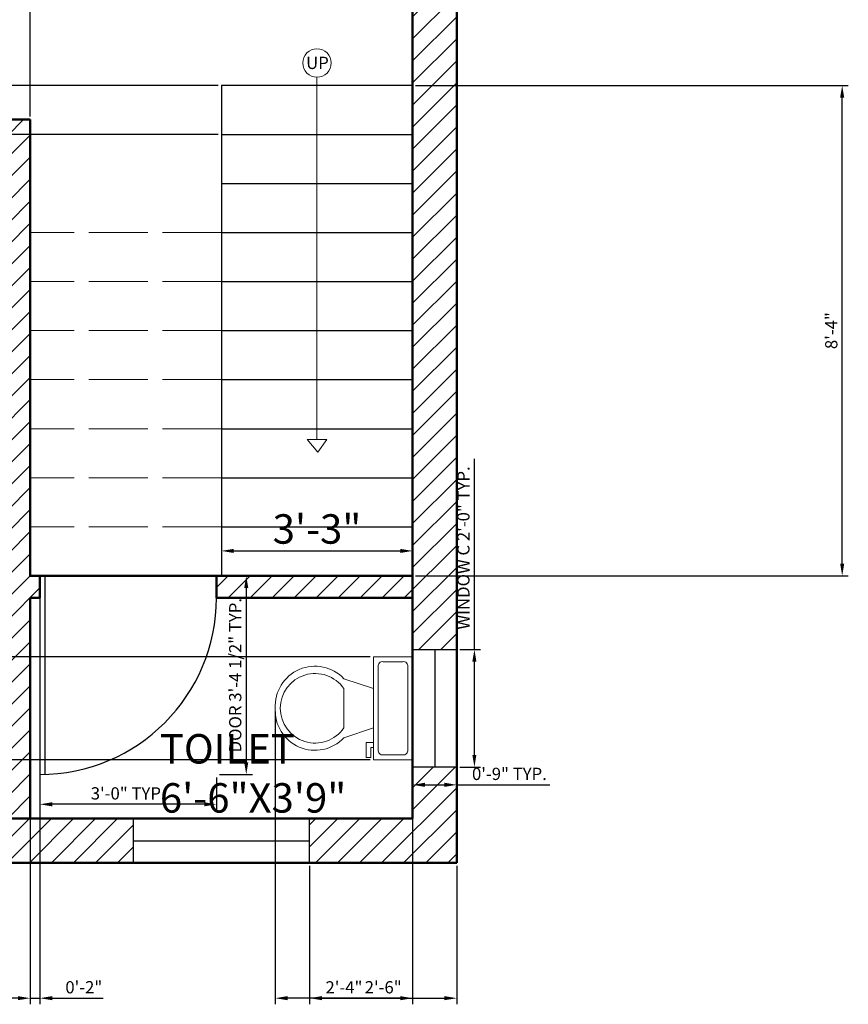
# Model space of a CAD drawing. Units: inches. Extents: x 3064 to 3516, y 2736 to 3280.
# Tile 2 of 5: x 3346 to 3515, y 2740 to 2941. Entities that reach past the tile are written whole.
import ezdxf

# ---------------------------------------------------------------- set-up
doc = ezdxf.new("R2010")
doc.units = ezdxf.units.IN
doc.linetypes.add('ACAD_ISO02W100', pattern=[15, 12, -3])
for name, color, linetype, lineweight in [('A-ANNO-DIMS', 2, 'Continuous', 18), ('A-ANNO-SYMB', 7, 'Continuous', 18), ('A-AREA-IDEN', 6, 'Continuous', 25), ('A-DOOR', 3, 'Continuous', 25), ('A-FLOR-FIXT', 9, 'Continuous', 20), ('A-FLOR-STRS', 7, 'Continuous', 25), ('A-FLOR-STRS-HIDN', 7, 'ACAD_ISO02W100', 18), ('A-GLAZ', 5, 'Continuous', 25), ('A-WALL', 7, 'Continuous', 50), ('A-WALL-PATT', 8, 'Continuous', 13)]:
    doc.layers.add(name, color=color, linetype=linetype, lineweight=lineweight)
doc.styles.get("Standard").update_dxf_attribs({"font": 'arial.ttf'})
doc.dimstyles.new('ISO-25', dxfattribs={"dimtxt": 2.5, "dimasz": 2.5, "dimexe": 1.25, "dimexo": 0.625, "dimtad": 1, "dimlunit": 3, "dimtxsty": 'Standard', "dimcen": 2.5, "dimadec": 0, "dimazin": 0, "dimtfac": 1, "dimtmove": 0, "dimatfit": 3, "dimfxl": 1, "dimarcsym": 0})

# ---------------------------------------------------------------- blocks, each defined once
blk = doc.blocks.new('*D1')
at = {"layer": 'A-ANNO-DIMS', "color": 0, "lineweight": -2, "transparency": 16777216}
for p, q in [((3387.4, 2832.69), (3387.4, 2831.35)), ((3389.9, 2832.6), (3423.9, 2832.6)), ((3426.4, 2832.69), (3426.4, 2831.35))]:
    blk.add_line(p, q, dxfattribs=at)
at = {"layer": 'A-ANNO-DIMS', "color": 0, "transparency": 16777216}
for points in [[(3389.9, 2833.01), (3389.9, 2832.18), (3387.4, 2832.6)], [(3423.9, 2833.01), (3423.9, 2832.18), (3426.4, 2832.6)]]:
    blk.add_solid(points, dxfattribs=at)
at = {"layer": 'Defpoints', "color": 0, "transparency": 16777216}
for p in [(3387.4, 2833.32), (3426.4, 2833.32), (3426.4, 2832.6)]:
    blk.add_point(p, dxfattribs=at)
at = {"layer": 'A-ANNO-DIMS', "color": 0, "transparency": 16777216, "insert": (3406.9, 2836.29), "char_height": 6, "attachment_point": 5}
blk.add_mtext('3\'-3"', dxfattribs=at)
blk = doc.blocks.new('*U6')
for p, q in [((9.5, -6), (9.5, -2)), ((-8, -8.5), (-8, -8)), ((-7, -8), (-7, -9.5)), ((-4, -8), (-6, -14)), ((4, -8), (6, -14)), ((-10, -8.5), (-8, -8.5)), ((-10, -9.5), (-10, -8.5)), ((-7, -9.5), (-10, -9.5)), ((4, -14), (-4, -14))]:
    blk.add_line(p, q)
blk.add_lwpolyline([(10.5, -8), (10.5, 0), (-10.5, 0), (-10.5, -8)], close=True)
for points in [[(-9.5, -2), (-9.5, -6)], [(8.5, -1), (-8.5, -1)], [(-8.5, -7), (8.5, -7)]]:
    blk.add_lwpolyline(points)
for centre, radius, start, end in [((-8.625, -1.875), 0.8839, 81.8699, 188.1301), ((8.625, -1.875), 0.8839, 351.8699, 98.1301), ((-8.625, -6.125), 0.8839, 171.869898, 278.1301), ((8.625, -6.125), 0.8839, 261.8699, 8.1301), ((-0.4772, -19.9188), 8.0953, 133.01722, 273.38), ((0.0374, -19.8731), 7.127, 124.50543, 269.7), ((-0.0373, -19.8731), 7.127, 270.3, 55.4946), ((0.4773, -19.9188), 8.0953, 266.62, 46.9828)]:
    blk.add_arc(centre, radius, start, end)
blk = doc.blocks.new('DOOR-SWING-36IN')
for p, q in [((-1, -4.5), (-1, 36)), ((0, 0), (0, 36))]:
    blk.add_line(p, q)
blk.add_arc((0, 0), 36, 90, 180)
blk = doc.blocks.new('WIN-36IN')
for p, q in [((36, 9), (0, 9)), ((0, 9), (0, 0)), ((36, 0), (36, 9)), ((0, 4.5), (36, 4.5)), ((0, 0), (36, 0))]:
    blk.add_line(p, q)
blk = doc.blocks.new('WIN-24IN')
for p, q in [((0, 24), (9, 24)), ((0, 0), (0, 24)), ((4.5, 24), (4.5, 0)), ((9, 24), (9, 0)), ((9, 0), (0, 0))]:
    blk.add_line(p, q)
blk = doc.blocks.new('*D17')
at = {"layer": 'A-ANNO-DIMS', "color": 0, "lineweight": -2, "transparency": 16777216}
for p, q in [((3387.02, 2827.51), (3393.72, 2827.51)), ((3392.47, 2825.01), (3392.47, 2789.51)), ((3387.02, 2787.01), (3393.72, 2787.01))]:
    blk.add_line(p, q, dxfattribs=at)
at = {"layer": 'A-ANNO-DIMS', "color": 0, "transparency": 16777216}
for points in [[(3392.06, 2825.01), (3392.89, 2825.01), (3392.47, 2827.51)], [(3392.06, 2789.51), (3392.89, 2789.51), (3392.47, 2787.01)]]:
    blk.add_solid(points, dxfattribs=at)
at = {"layer": 'Defpoints', "color": 0, "transparency": 16777216}
for p in [(3386.4, 2827.51), (3386.4, 2787.01), (3392.47, 2787.01)]:
    blk.add_point(p, dxfattribs=at)
at = {"layer": 'A-ANNO-DIMS', "color": 0, "transparency": 16777216, "insert": (3390.55, 2807.26), "char_height": 2.5, "attachment_point": 5, "rotation": 90}
blk.add_mtext('DOOR 3\'-4 1/2" TYP.', dxfattribs=at)
blk = doc.blocks.new('*D18')
at = {"layer": 'A-ANNO-DIMS', "color": 0, "lineweight": -2, "transparency": 16777216}
for p, q in [((3350.4, 2786.39), (3350.4, 2779.69)), ((3386.4, 2786.39), (3386.4, 2779.69)), ((3383.9, 2780.94), (3352.9, 2780.94))]:
    blk.add_line(p, q, dxfattribs=at)
at = {"layer": 'A-ANNO-DIMS', "color": 0, "transparency": 16777216}
for points in [[(3352.9, 2781.36), (3352.9, 2780.52), (3350.4, 2780.94)], [(3383.9, 2781.36), (3383.9, 2780.52), (3386.4, 2780.94)]]:
    blk.add_solid(points, dxfattribs=at)
at = {"layer": 'Defpoints', "color": 0, "transparency": 16777216}
for p in [(3350.4, 2787.01), (3386.4, 2787.01), (3350.4, 2780.94)]:
    blk.add_point(p, dxfattribs=at)
at = {"layer": 'A-ANNO-DIMS', "color": 0, "transparency": 16777216, "insert": (3368.4, 2782.84), "char_height": 2.5, "attachment_point": 5}
blk.add_mtext('3\'-0" TYP.', dxfattribs=at)
blk = doc.blocks.new('*D23')
at = {"layer": 'A-ANNO-DIMS', "color": 0, "lineweight": -2, "transparency": 16777216}
for p, q in [((3439, 2812.51), (3439, 2851.39)), ((3436.02, 2812.51), (3440.25, 2812.51)), ((3439, 2791.01), (3439, 2810.01)), ((3436.02, 2788.51), (3440.25, 2788.51))]:
    blk.add_line(p, q, dxfattribs=at)
at = {"layer": 'A-ANNO-DIMS', "color": 0, "transparency": 16777216}
for points in [[(3438.58, 2810.01), (3439.41, 2810.01), (3439, 2812.51)], [(3438.58, 2791.01), (3439.41, 2791.01), (3439, 2788.51)]]:
    blk.add_solid(points, dxfattribs=at)
at = {"layer": 'Defpoints', "color": 0, "transparency": 16777216}
for p in [(3435.4, 2812.51), (3439, 2812.51), (3435.4, 2788.51)]:
    blk.add_point(p, dxfattribs=at)
at = {"layer": 'A-ANNO-DIMS', "color": 0, "transparency": 16777216, "insert": (3437.08, 2833.2), "char_height": 2.5, "attachment_point": 5, "rotation": 90}
blk.add_mtext('WINDOW C 2\'-0" TYP.', dxfattribs=at)
blk = doc.blocks.new('*D24')
at = {"layer": 'A-ANNO-DIMS', "color": 0, "lineweight": -2, "transparency": 16777216}
for p, q in [((3426.4, 2787.89), (3426.4, 2783.66)), ((3435.4, 2787.89), (3435.4, 2783.66)), ((3428.9, 2784.91), (3432.9, 2784.91)), ((3435.4, 2784.91), (3454.39, 2784.91))]:
    blk.add_line(p, q, dxfattribs=at)
at = {"layer": 'A-ANNO-DIMS', "color": 0, "transparency": 16777216}
for points in [[(3428.9, 2785.33), (3428.9, 2784.5), (3426.4, 2784.91)], [(3432.9, 2785.33), (3432.9, 2784.5), (3435.4, 2784.91)]]:
    blk.add_solid(points, dxfattribs=at)
at = {"layer": 'Defpoints', "color": 0, "transparency": 16777216}
for p in [(3426.4, 2788.51), (3435.4, 2788.51), (3435.4, 2784.91)]:
    blk.add_point(p, dxfattribs=at)
at = {"layer": 'A-ANNO-DIMS', "color": 0, "transparency": 16777216, "insert": (3446.14, 2786.82), "char_height": 2.5, "attachment_point": 5}
blk.add_mtext('0\'-9" TYP.', dxfattribs=at)
blk = doc.blocks.new('*D43')
at = {"layer": 'A-ANNO-DIMS', "color": 0, "lineweight": -2, "transparency": 16777216}
for p, q in [((3405.4, 2768.39), (3405.4, 2740.16)), ((3435.4, 2768.39), (3435.4, 2740.16)), ((3407.9, 2741.41), (3432.9, 2741.41))]:
    blk.add_line(p, q, dxfattribs=at)
at = {"layer": 'A-ANNO-DIMS', "color": 0, "transparency": 16777216}
for points in [[(3407.9, 2741.83), (3407.9, 2741), (3405.4, 2741.41)], [(3432.9, 2741.83), (3432.9, 2741), (3435.4, 2741.41)]]:
    blk.add_solid(points, dxfattribs=at)
at = {"layer": 'Defpoints', "color": 0, "transparency": 16777216}
for p in [(3405.4, 2769.01), (3435.4, 2769.01), (3435.4, 2741.41)]:
    blk.add_point(p, dxfattribs=at)
at = {"layer": 'A-ANNO-DIMS', "color": 0, "transparency": 16777216, "insert": (3420.4, 2743.32), "char_height": 2.5, "attachment_point": 5}
blk.add_mtext('2\'-6"', dxfattribs=at)
blk = doc.blocks.new('*D44')
at = {"layer": 'A-ANNO-DIMS', "color": 0, "lineweight": -2, "transparency": 16777216}
for p, q in [((3343.9, 2921.14), (3343.9, 3240.36)), ((3348.4, 2921.14), (3348.4, 3240.36)), ((3341.4, 3239.11), (3325.18, 3239.11)), ((3348.4, 3239.11), (3343.9, 3239.11)), ((3350.9, 3239.11), (3353.4, 3239.11))]:
    blk.add_line(p, q, dxfattribs=at)
at = {"layer": 'A-ANNO-DIMS', "color": 0, "transparency": 16777216}
for points in [[(3341.4, 3239.53), (3341.4, 3238.7), (3343.9, 3239.11)], [(3350.9, 3239.53), (3350.9, 3238.7), (3348.4, 3239.11)]]:
    blk.add_solid(points, dxfattribs=at)
at = {"layer": 'Defpoints', "color": 0, "transparency": 16777216}
for p in [(3343.9, 3239.11), (3343.9, 2920.51), (3348.4, 2920.51)]:
    blk.add_point(p, dxfattribs=at)
at = {"layer": 'A-ANNO-DIMS', "color": 0, "transparency": 16777216, "insert": (3332.04, 3241.03), "char_height": 2.5, "attachment_point": 5}
blk.add_mtext('0\'-4 1/2"', dxfattribs=at)
blk = doc.blocks.new('*D45')
at = {"layer": 'A-ANNO-DIMS', "color": 0, "lineweight": -2, "transparency": 16777216}
for p, q in [((3386.77, 2927.51), (3068.05, 2927.51)), ((3069.3, 2925.01), (3069.3, 2920.01)), ((3386.77, 2917.51), (3068.05, 2917.51))]:
    blk.add_line(p, q, dxfattribs=at)
at = {"layer": 'A-ANNO-DIMS', "color": 0, "transparency": 16777216}
for points in [[(3068.88, 2925.01), (3069.71, 2925.01), (3069.3, 2927.51)], [(3068.88, 2920.01), (3069.71, 2920.01), (3069.3, 2917.51)]]:
    blk.add_solid(points, dxfattribs=at)
at = {"layer": 'Defpoints', "color": 0, "transparency": 16777216}
for p in [(3387.4, 2927.51), (3069.3, 2917.51), (3387.4, 2917.51)]:
    blk.add_point(p, dxfattribs=at)
at = {"layer": 'A-ANNO-DIMS', "color": 0, "transparency": 16777216, "insert": (3067.4, 2922.51), "char_height": 2.5, "attachment_point": 5, "rotation": 90}
blk.add_mtext('0\'-10"', dxfattribs=at)
blk = doc.blocks.new('*D46')
at = {"layer": 'A-ANNO-DIMS', "color": 0, "lineweight": -2, "transparency": 16777216}
for p, q in [((3427.02, 2927.51), (3515.25, 2927.51)), ((3514, 2830.01), (3514, 2925.01)), ((3427.02, 2827.51), (3515.25, 2827.51))]:
    blk.add_line(p, q, dxfattribs=at)
at = {"layer": 'A-ANNO-DIMS', "color": 0, "transparency": 16777216}
for points in [[(3513.58, 2925.01), (3514.41, 2925.01), (3514, 2927.51)], [(3513.58, 2830.01), (3514.41, 2830.01), (3514, 2827.51)]]:
    blk.add_solid(points, dxfattribs=at)
at = {"layer": 'Defpoints', "color": 0, "transparency": 16777216}
for p in [(3426.4, 2927.51), (3514, 2927.51), (3426.4, 2827.51)]:
    blk.add_point(p, dxfattribs=at)
at = {"layer": 'A-ANNO-DIMS', "color": 0, "transparency": 16777216, "insert": (3512.1, 2877.51), "char_height": 2.5, "attachment_point": 5, "rotation": 90}
blk.add_mtext('8\'-4"', dxfattribs=at)
blk = doc.blocks.new('*D48')
at = {"layer": 'A-ANNO-DIMS', "color": 0, "lineweight": -2, "transparency": 16777216}
for p, q in [((3417.77, 2811.01), (3068.05, 2811.01)), ((3069.3, 2808.51), (3069.3, 2792.51)), ((3417.77, 2790.01), (3068.05, 2790.01))]:
    blk.add_line(p, q, dxfattribs=at)
at = {"layer": 'A-ANNO-DIMS', "color": 0, "transparency": 16777216}
for points in [[(3068.88, 2808.51), (3069.71, 2808.51), (3069.3, 2811.01)], [(3068.88, 2792.51), (3069.71, 2792.51), (3069.3, 2790.01)]]:
    blk.add_solid(points, dxfattribs=at)
at = {"layer": 'Defpoints', "color": 0, "transparency": 16777216}
for p in [(3418.4, 2811.01), (3069.3, 2790.01), (3418.4, 2790.01)]:
    blk.add_point(p, dxfattribs=at)
at = {"layer": 'A-ANNO-DIMS', "color": 0, "transparency": 16777216, "insert": (3067.4, 2800.51), "char_height": 2.5, "attachment_point": 5, "rotation": 90}
blk.add_mtext('1\'-9"', dxfattribs=at)
blk = doc.blocks.new('*D49')
at = {"layer": 'A-ANNO-DIMS', "color": 0, "lineweight": -2, "transparency": 16777216}
for p, q in [((3398.4, 2799.89), (3398.4, 2740.16)), ((3426.4, 2789.39), (3426.4, 2740.16)), ((3423.9, 2741.41), (3400.9, 2741.41))]:
    blk.add_line(p, q, dxfattribs=at)
at = {"layer": 'A-ANNO-DIMS', "color": 0, "transparency": 16777216}
for points in [[(3400.9, 2741.83), (3400.9, 2741), (3398.4, 2741.41)], [(3423.9, 2741.83), (3423.9, 2741), (3426.4, 2741.41)]]:
    blk.add_solid(points, dxfattribs=at)
at = {"layer": 'Defpoints', "color": 0, "transparency": 16777216}
for p in [(3398.4, 2800.51), (3426.4, 2790.01), (3398.4, 2741.41)]:
    blk.add_point(p, dxfattribs=at)
at = {"layer": 'A-ANNO-DIMS', "color": 0, "transparency": 16777216, "insert": (3412.4, 2743.3), "char_height": 2.5, "attachment_point": 5}
blk.add_mtext('2\'-4"', dxfattribs=at)
blk = doc.blocks.new('*D63')
at = {"layer": 'A-ANNO-DIMS', "color": 0, "lineweight": -2, "transparency": 16777216}
for p, q in [((3348.4, 2822.39), (3348.4, 2740.16)), ((3350.4, 2822.39), (3350.4, 2740.16)), ((3345.9, 2741.41), (3343.4, 2741.41)), ((3348.4, 2741.41), (3350.4, 2741.41)), ((3352.9, 2741.41), (3363.29, 2741.41))]:
    blk.add_line(p, q, dxfattribs=at)
at = {"layer": 'A-ANNO-DIMS', "color": 0, "transparency": 16777216}
for points in [[(3345.9, 2741.83), (3345.9, 2741), (3348.4, 2741.41)], [(3352.9, 2741.83), (3352.9, 2741), (3350.4, 2741.41)]]:
    blk.add_solid(points, dxfattribs=at)
at = {"layer": 'Defpoints', "color": 0, "transparency": 16777216}
for p in [(3348.4, 2823.01), (3350.4, 2823.01), (3350.4, 2741.41)]:
    blk.add_point(p, dxfattribs=at)
at = {"layer": 'A-ANNO-DIMS', "color": 0, "transparency": 16777216, "insert": (3359.35, 2743.32), "char_height": 2.5, "attachment_point": 5}
blk.add_mtext('0\'-2"', dxfattribs=at)

msp = doc.modelspace()

# ---------------------------------------------------------------- hatches: boundary and pattern name
at = {"layer": 'A-WALL-PATT'}
h = msp.add_hatch(dxfattribs=at)
h.set_pattern_fill('ANSI31', color=256)
h.paths.add_polyline_path([(3156.897, 2985.015), (3147.897, 2985.015), (3147.897, 2923.515), (3156.897, 2923.515)])
h.paths.add_polyline_path([(3156.897, 2863.515), (3147.897, 2863.515), (3147.897, 2812.515), (3156.897, 2812.515)])
h.paths.add_polyline_path([(3293.397, 2778.015), (3239.397, 2778.015), (3239.397, 2780.015), (3234.897, 2780.015), (3234.897, 2778.015), (3156.897, 2778.015), (3156.897, 2788.515), (3147.897, 2788.515), (3147.897, 2769.015), (3293.397, 2769.015)])
h.paths.add_polyline_path([(3369.397, 2778.015), (3343.897, 2778.015), (3344.15, 2769.015), (3369.397, 2769.015)])
h.paths.add_polyline_path([(3435.397, 2788.515), (3426.397, 2788.515), (3426.397, 2778.015), (3405.397, 2778.015), (3405.397, 2769.015), (3435.397, 2769.015)])
h.paths.add_polyline_path([(3435.397, 2960.265), (3426.397, 2960.265), (3426.397, 2812.515), (3435.397, 2812.515)])
h.paths.add_polyline_path([(3435.397, 3094.515), (3426.397, 3094.515), (3426.397, 3020.265), (3435.397, 3020.265)])
h.paths.add_polyline_path([(3435.397, 3211.515), (3147.897, 3211.515), (3147.897, 3154.515), (3156.897, 3154.515), (3156.897, 3202.515), (3426.397, 3202.515), (3426.397, 3154.515), (3435.397, 3154.515)])
h.paths.add_polyline_path([(3293.397, 3202.515), (3288.897, 3202.515), (3288.897, 3046.515), (3285.897, 3046.515), (3285.897, 3042.015), (3296.397, 3042.015), (3296.397, 3046.515), (3293.397, 3046.515)])
h.paths.add_polyline_path([(3426.397, 3046.515), (3332.397, 3046.515), (3332.397, 3042.015), (3426.397, 3042.015)])
h.paths.add_polyline_path([(3249.897, 3046.515), (3156.897, 3046.515), (3156.897, 3042.015), (3249.897, 3042.015)])
h.paths.add_polyline_path([(3156.897, 3094.515), (3147.897, 3094.515), (3147.897, 3021.015), (3156.897, 3021.015)])
h.paths.add_polyline_path([(3293.397, 2964.015), (3156.897, 2964.015), (3156.897, 2959.515), (3288.897, 2959.515), (3288.897, 2956.515), (3293.397, 2956.515)])
h.paths.add_polyline_path([(3249.897, 2827.515), (3156.897, 2827.515), (3156.897, 2823.015), (3234.897, 2823.015), (3234.897, 2816.015), (3239.397, 2816.015), (3239.397, 2823.015), (3249.897, 2823.015)])
h.paths.add_polyline_path([(3293.397, 2920.515), (3288.897, 2920.515), (3288.897, 2827.515), (3285.897, 2827.515), (3285.897, 2823.015), (3293.397, 2823.015), (3293.397, 2856.015), (3305.897, 2856.015), (3305.897, 2860.515), (3293.397, 2860.515)])
h.paths.add_polyline_path([(3348.397, 2920.515), (3343.897, 2920.515), (3343.897, 2860.515), (3341.897, 2860.515), (3341.897, 2856.015), (3343.897, 2856.015), (3343.897, 2778.015), (3348.397, 2778.015), (3348.397, 2823.015), (3350.397, 2823.015), (3350.397, 2827.515), (3348.397, 2827.515)])
h.paths.add_polyline_path([(3426.397, 2827.515), (3386.397, 2827.515), (3386.397, 2823.015), (3426.397, 2823.015)])

# ---------------------------------------------------------------- linework, layer by layer
at = {"layer": 'A-ANNO-SYMB'}
for p, q in [((3406.897, 2929.176), (3406.897, 2857.515)), ((3406.897, 2857.515), (3406.897, 2855.318)), ((3406.897, 2855.318), (3404.887, 2855.318)), ((3404.887, 2855.318), (3407.079, 2852.73)), ((3406.897, 2855.318), (3408.907, 2855.318)), ((3408.907, 2855.318), (3407.079, 2852.73))]:
    msp.add_line(p, q, dxfattribs=at)
msp.add_circle((3406.897, 2932.071), 2.895, dxfattribs=at)
at = {"layer": 'A-FLOR-STRS'}
for p, q in [((3387.397, 2927.515), (3387.397, 2827.515)), ((3387.397, 2927.515), (3426.397, 2927.515)), ((3387.397, 2917.515), (3426.397, 2917.515)), ((3387.397, 2907.515), (3426.397, 2907.515)), ((3387.397, 2897.515), (3426.397, 2897.515)), ((3387.397, 2887.515), (3426.397, 2887.515)), ((3387.397, 2877.515), (3426.397, 2877.515)), ((3387.397, 2867.515), (3426.397, 2867.515)), ((3387.397, 2857.515), (3426.397, 2857.515)), ((3387.397, 2847.515), (3426.397, 2847.515)), ((3387.397, 2837.515), (3426.397, 2837.515))]:
    msp.add_line(p, q, dxfattribs=at)
at = {"layer": 'A-FLOR-STRS-HIDN'}
for p, q in [((3387.397, 2897.515), (3348.397, 2897.515)), ((3387.397, 2887.515), (3348.397, 2887.515)), ((3387.397, 2877.515), (3348.397, 2877.515)), ((3387.397, 2867.515), (3348.397, 2867.515)), ((3387.397, 2857.515), (3348.397, 2857.515)), ((3387.397, 2847.515), (3348.397, 2847.515)), ((3387.397, 2837.515), (3348.397, 2837.515))]:
    msp.add_line(p, q, dxfattribs=at)
at = {"layer": 'A-WALL'}
for p, q in [((3435.397, 3211.515), (3435.397, 2769.015)), ((3426.397, 3202.515), (3426.397, 2778.015)), ((3343.897, 2920.515), (3348.397, 2920.515)), ((3348.397, 2920.515), (3348.397, 2827.515)), ((3348.397, 2827.515), (3426.397, 2827.515)), ((3348.397, 2827.515), (3350.397, 2827.515)), ((3350.397, 2827.515), (3350.397, 2823.015)), ((3386.397, 2823.015), (3386.397, 2827.515)), ((3348.397, 2823.015), (3350.397, 2823.015)), ((3348.397, 2823.015), (3348.397, 2778.015)), ((3386.397, 2823.015), (3426.397, 2823.015)), ((3239.397, 2778.015), (3426.397, 2778.015)), ((3147.897, 2769.015), (3435.397, 2769.015))]:
    msp.add_line(p, q, dxfattribs=at)

# ---------------------------------------------------------------- block references
at = {"layer": 'A-DOOR', "rotation": 180}
msp.add_blockref('DOOR-SWING-36IN', (3350.397, 2823.015), dxfattribs=at)
at = {"layer": 'A-FLOR-FIXT', "xscale": -1, "rotation": 270}
msp.add_blockref('*U6', (3426.397, 2800.515), dxfattribs=at)
at = {"layer": 'A-GLAZ'}
for name, p in [('WIN-24IN', (3426.397, 2788.515)), ('WIN-36IN', (3369.397, 2769.015))]:
    msp.add_blockref(name, p, dxfattribs=at)

# ---------------------------------------------------------------- texts
at = {"layer": 'A-ANNO-SYMB', "insert": (3404.685, 2933.342), "char_height": 2.5, "attachment_point": 1}
msp.add_mtext_dynamic_manual_height_columns('UP', width=2.68506, gutter_width=12.5, heights=[0], dxfattribs=at)
at = {"layer": 'A-AREA-IDEN', "insert": (3374.861, 2795.25), "char_height": 6, "attachment_point": 1}
msp.add_mtext_dynamic_manual_height_columns('TOILET\\P6\'-6"X3\'9"', width=17.38334, gutter_width=12.5, heights=[0], dxfattribs=at)

# ---------------------------------------------------------------- dimensions: what is measured, and where the dimension line sits
at = {"layer": 'A-ANNO-DIMS'}
for base, p1, p2, override, picture, middle in [((3343.897, 3239.115), (3348.397, 2920.515), (3343.897, 2920.515), {"dimdec": 1, "dimlfac": 1, "dimrnd": 0, "dimzin": 1, "dimdsep": 46, "dimlunit": 4, "dimfrac": 2}, '*D44', (3332.037, 3241.033)), ((3426.397, 2832.595), (3387.397, 2833.317), (3426.397, 2833.317), {"dimtxt": 6, "dimclrd": 0, "dimclre": 0, "dimclrt": 0}, '*D1', (3406.897, 2836.286)), ((3350.397, 2741.415), (3348.397, 2823.015), (3350.397, 2823.015), {"dimdec": 1, "dimlfac": 1, "dimrnd": 0, "dimzin": 1, "dimdsep": 46, "dimlunit": 4, "dimfrac": 2}, '*D63', (3359.345, 2743.316)), ((3398.397, 2741.415), (3426.397, 2790.015), (3398.397, 2800.515), {"dimdec": 1, "dimlfac": 1, "dimrnd": 0, "dimzin": 1, "dimdsep": 46, "dimlunit": 4, "dimfrac": 2}, '*D49', (3412.397, 2743.295)), ((3435.397, 2741.415), (3405.397, 2769.015), (3435.397, 2769.015), {"dimdec": 1, "dimlfac": 1, "dimrnd": 0, "dimzin": 1, "dimdsep": 46, "dimlunit": 4, "dimfrac": 2}, '*D43', (3420.397, 2743.316))]:
    dim = msp.add_linear_dim(base=base, p1=p1, p2=p2, dimstyle='ISO-25', override=override, dxfattribs=at)
    dim.commit()
    dim.dimension.update_dxf_attribs({"geometry": picture, "text_midpoint": middle})
for base, p1, p2, picture, middle in [((3069.297, 2917.515), (3387.397, 2927.515), (3387.397, 2917.515), '*D45', (3067.396, 2922.515)), ((3513.997, 2927.515), (3426.397, 2827.515), (3426.397, 2927.515), '*D46', (3512.096, 2877.515)), ((3069.297, 2790.015), (3418.397, 2811.015), (3418.397, 2790.015), '*D48', (3067.396, 2800.515))]:
    dim = msp.add_linear_dim(base=base, p1=p1, p2=p2, angle=90, dimstyle='ISO-25', override={"dimdec": 1, "dimlfac": 1, "dimrnd": 0, "dimzin": 1, "dimdsep": 46, "dimlunit": 4, "dimfrac": 2}, dxfattribs=at)
    dim.commit()
    dim.dimension.update_dxf_attribs({"geometry": picture, "text_midpoint": middle})
for base, p1, p2, angle, text, picture, middle in [((3438.997, 2812.515), (3435.397, 2788.515), (3435.397, 2812.515), 90, 'WINDOW C <> TYP.', '*D23', (3437.079, 2833.204)), ((3392.472, 2787.015), (3386.397, 2827.515), (3386.397, 2787.015), 270, 'DOOR <> TYP.', '*D17', (3390.553, 2807.265)), ((3350.397, 2780.94), (3386.397, 2787.015), (3350.397, 2787.015), 180, '<> TYP.', '*D18', (3368.397, 2782.842))]:
    dim = msp.add_linear_dim(base=base, p1=p1, p2=p2, angle=angle, text=text, dimstyle='ISO-25', override={"dimdec": 1, "dimlfac": 1, "dimrnd": 0, "dimzin": 1, "dimdsep": 46, "dimlunit": 4, "dimfrac": 2}, dxfattribs=at)
    dim.commit()
    dim.dimension.update_dxf_attribs({"geometry": picture, "text_midpoint": middle})
dim = msp.add_linear_dim(base=(3435.397, 2784.915), p1=(3426.397, 2788.515), p2=(3435.397, 2788.515), text='<> TYP.', dimstyle='ISO-25', override={"dimdec": 1, "dimlfac": 1, "dimrnd": 0, "dimzin": 1, "dimdsep": 46, "dimlunit": 4, "dimfrac": 2}, dxfattribs=at)
dim.commit()
dim.dimension.update_dxf_attribs({"geometry": '*D24', "text_midpoint": (3446.142, 2786.816)})

doc.saveas('drawing.dxf')
